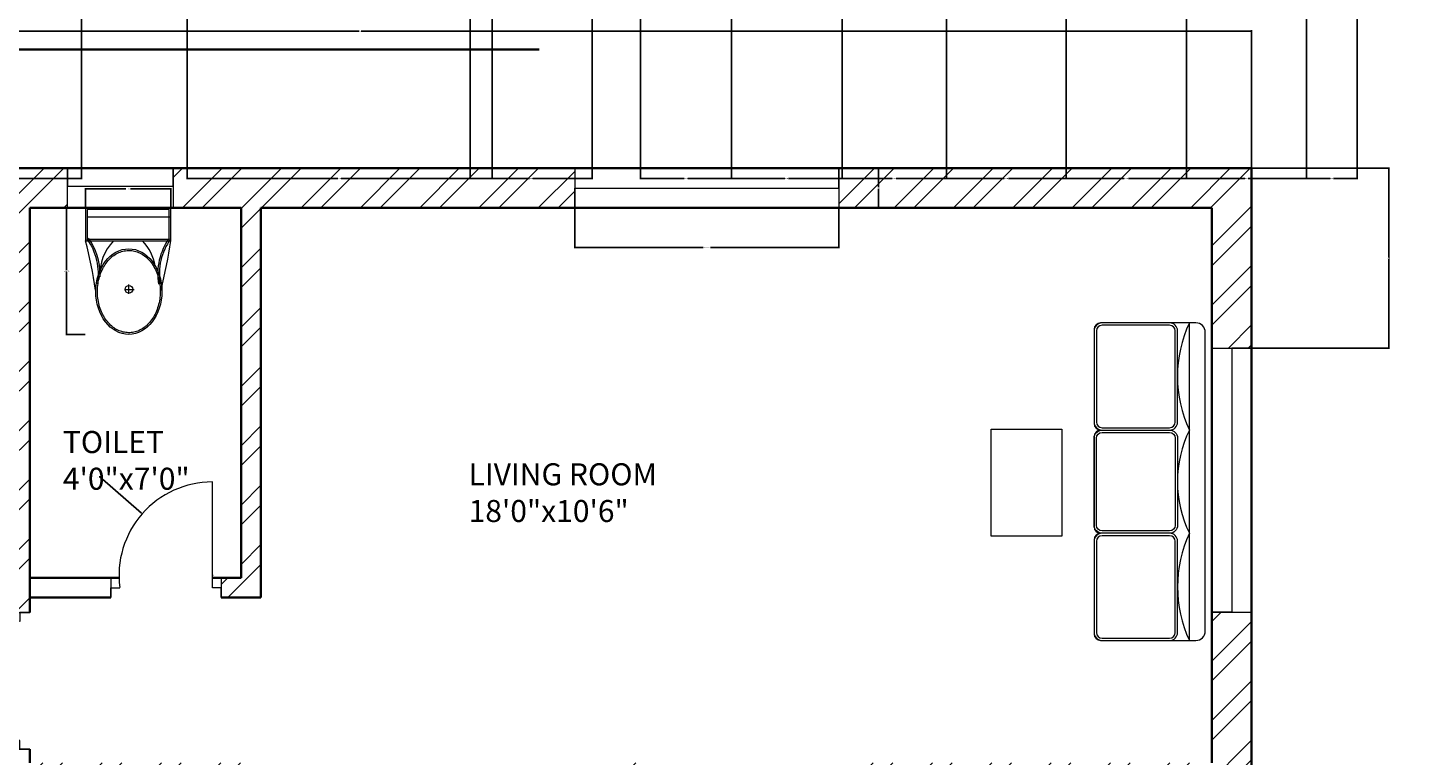
# Model space of a CAD drawing. Units: inches. Extents: x 1955 to 3324, y 980 to 3129.
# Tile 6 of 11: x 2237 to 2555, y 2323 to 2488. Entities that reach past the tile are written whole.
import ezdxf

# ---------------------------------------------------------------- set-up
doc = ezdxf.new("R2010")
doc.units = ezdxf.units.IN
for name, color, linetype, lineweight in [('A-ANNO-DIMS', 2, 'Continuous', 18), ('A-ANNO-TITL', 7, 'Continuous', 35), ('A-AREA-IDEN', 7, 'Continuous', 18), ('A-DOOR', 3, 'Continuous', 18), ('A-FLOR-FIXT', 9, 'Continuous', 18), ('A-FURN', 8, 'Continuous', 18), ('A-GLAZ', 4, 'Continuous', 18), ('A-WALL', 7, 'Continuous', 35), ('A-WALL-PATT', 252, 'Continuous', 13)]:
    doc.layers.add(name, color=color, linetype=linetype, lineweight=lineweight)
doc.styles.get("Standard").update_dxf_attribs({"font": 'arial.ttf'})
doc.dimstyles.get("Standard").update_dxf_attribs({"dimtxt": 0.18, "dimasz": 0.18, "dimexe": 0.18, "dimexo": 0.0625, "dimgap": 0.09, "dimtad": 0, "dimtih": 1, "dimtoh": 1, "dimdec": 4, "dimzin": 0, "dimdsep": 46, "dimtxsty": 'Standard', "dimcen": 0.09, "dimadec": 0, "dimazin": 0, "dimtfac": 1, "dimtdec": 4, "dimtofl": 0, "dimtmove": 0, "dimatfit": 3, "dimfxl": 1, "dimtolj": 1, "dimtzin": 0, "dimarcsym": 0})

# ---------------------------------------------------------------- blocks, each defined once
blk = doc.blocks.new('A$C31115884')
for p, q in [((257.5, 466.4), (257.5, 523.2)), ((283.1, 497.7), (223.4, 497.7)), ((0, 200), (0, 0)), ((520, 200), (0, 200)), ((10, 190), (10, 10)), ((510, 190), (10, 190)), ((510, 10), (510, 190)), ((520, 0), (520, 200)), ((510, 54.5), (0, 54.5)), ((10, 10), (510, 10)), ((0, 0), (520, 0))]:
    blk.add_line(p, q)
blk.add_circle((255.6, 496.4), 23.6)
for centre, radius, start, end in [((2777.7, -204.6), 2807, 165.4549, 171.71327), ((-294.5, 403.3), 364.7, 324.20913, 9.34987), ((-294.5, 403.3), 374.7, 324.20913, 9.34987), ((805.8, 403.3), 364.7, 170.65013, 215.79087), ((3237, 905), 2807, 188.28673, 194.5451), ((383.6, 406.2), 293.5, 190.27735, 224.15636), ((139.5, 406.2), 293.5, 315.84364, 2.65635), ((805.8, 403.3), 374.7, 179.20365, 215.79087)]:
    blk.add_arc(centre, radius, start, end)
blk.add_ellipse((256.2, 509.9), major_axis=(0, -260.7), ratio=0.772727)
blk.add_open_spline([(256.2, 259.2), (263.1, 259.2), (270, 259.7), (287.8, 262.3), (298.7, 265.1), (319.9, 273.1), (330.2, 278.4), (350.1, 291.1), (359.7, 298.7), (377.7, 315.9), (386.2, 325.5), (401.7, 346.6), (408.8, 358.1), (421.3, 382.5), (426.8, 395.5), (435.9, 422.4), (439.5, 436.4), (444.8, 465.1), (446.5, 479.7), (447.9, 509.2), (447.6, 524), (445, 553.3), (442.7, 567.8), (436.3, 596), (432.1, 609.7), (421.9, 636), (416, 648.6), (402.5, 672.1), (395, 683), (378.6, 703), (369.8, 712.1), (351.1, 728), (341.3, 734.8), (320.9, 746.2), (310.4, 750.7), (288.9, 757.3), (278, 759.4), (256, 761), (245, 760.6), (223.1, 757.2), (212.3, 754.3), (191.1, 746.1), (180.8, 740.7), (160.9, 727.8), (151.4, 720.1), (133.5, 702.7), (125.1, 693), (109.6, 671.7), (102.6, 660.2), (90.2, 635.7), (84.9, 622.7), (76, 595.6), (72.4, 581.6), (67.2, 552.9), (65.6, 538.2), (64.4, 508.8), (64.8, 494), (67.5, 464.7), (69.9, 450.2), (76.6, 422), (80.8, 408.3), (91.1, 382.2), (97.2, 369.7), (110.8, 346.3), (118.4, 335.4), (134.8, 315.6), (143.7, 306.7), (162.4, 290.9), (172.3, 284.2), (192.8, 273), (203.3, 268.6), (224.8, 262.2), (235.8, 260.2), (249.9, 259.3), (253, 259.2), (256.2, 259.2)], degree=3, knots=[0, 0, 0, 0, 0.110105, 0.110105, 0.285049, 0.285049, 0.459994, 0.459994, 0.634938, 0.634938, 0.809882, 0.809882, 0.984827, 0.984827, 1.159771, 1.159771, 1.334715, 1.334715, 1.50966, 1.50966, 1.684604, 1.684604, 1.859549, 1.859549, 2.034493, 2.034493, 2.209437, 2.209437, 2.384382, 2.384382, 2.559326, 2.559326, 2.73427, 2.73427, 2.909215, 2.909215, 3.084159, 3.084159, 3.259103, 3.259103, 3.434048, 3.434048, 3.608992, 3.608992, 3.783936, 3.783936, 3.958881, 3.958881, 4.133825, 4.133825, 4.30877, 4.30877, 4.483714, 4.483714, 4.658658, 4.658658, 4.833603, 4.833603, 5.008547, 5.008547, 5.183491, 5.183491, 5.358436, 5.358436, 5.53338, 5.53338, 5.708324, 5.708324, 5.883269, 5.883269, 6.058213, 6.058213, 6.233158, 6.233158, 6.283185, 6.283185, 6.283185, 6.283185])
blk = doc.blocks.new('COFFEE-TABLE-RECT')
blk.add_lwpolyline([(0, 24.35), (16.02, 24.35), (16.02, 0), (0, 0)], close=True)
blk = doc.blocks.new('DOOR-BED-N')
for p, q in [((33.75, 31.05), (38.25, 31.05)), ((38.25, 31.05), (36, 31.05)), ((36, 31.05), (36, 29.05)), ((36, 2), (0, 2)), ((36, 0), (36, 2)), ((33.75, 0), (38.25, 0)), ((38.25, 0), (36, 0))]:
    blk.add_line(p, q)
blk.add_arc((28.16, 2), 28.16, 73.8433, 180)
blk = doc.blocks.new('DOOR-WC-N')
for p, q in [((23.02, 2.25), (23.02, 26.25)), ((0, 4.5), (0, 0)), ((25.02, 4.5), (25.02, 0)), ((0, 0), (0, 2.25)), ((0, 2.25), (2, 2.25)), ((25.02, 2.25), (23.02, 2.25)), ((25.02, 0), (25.02, 2.25))]:
    blk.add_line(p, q)
blk.add_arc((23.02, 5.05), 21.2, 90, 187.5818)
blk = doc.blocks.new('WIN-PLAN-60-A')
for p, q in [((0, 60), (9, 60)), ((9, 60), (4.5, 60)), ((4.5, 60), (4.5, 0)), ((4.5, 0), (0, 0)), ((0, 0), (9, 0))]:
    blk.add_line(p, q)
blk = doc.blocks.new('WIN-PLAN-60-C')
for p, q in [((0, 9), (0, 0)), ((60, 4.5), (60, 9)), ((60, 9), (60, 9)), ((60, 9), (60, 0)), ((0, 0), (0, 4.5)), ((0, 4.5), (60, 4.5))]:
    blk.add_line(p, q)
blk = doc.blocks.new('WIN-PLAN-24-B')
for p, q in [((0, 0), (0, 9)), ((0, 9), (0, 4.93)), ((24, 4.93), (24, 9)), ((24, 9), (24, 0)), ((0, 4.93), (24, 4.93))]:
    blk.add_line(p, q)
blk = doc.blocks.new('*D35')
at = {"layer": 'A-ANNO-DIMS', "color": 0, "lineweight": -2, "transparency": 16777216}
for p, q in [((2361.48, 2447.44), (2361.48, 2438.32)), ((2421.48, 2447.44), (2421.48, 2438.32)), ((2361.66, 2438.5), (2390.63, 2438.5)), ((2421.3, 2438.5), (2392.32, 2438.5))]:
    blk.add_line(p, q, dxfattribs=at)
at = {"layer": 'A-ANNO-DIMS', "color": 0, "transparency": 16777216}
for points in [[(2361.66, 2438.53), (2361.66, 2438.47), (2361.48, 2438.5)], [(2421.3, 2438.53), (2421.3, 2438.47), (2421.48, 2438.5)]]:
    blk.add_solid(points, dxfattribs=at)
at = {"layer": 'Defpoints', "color": 0, "transparency": 16777216}
for p in [(2361.48, 2447.5), (2421.48, 2447.5), (2421.48, 2438.5)]:
    blk.add_point(p, dxfattribs=at)
at = {"layer": 'A-ANNO-DIMS', "color": 0, "transparency": 16777216, "insert": (2391.48, 2438.5), "char_height": 0.18, "attachment_point": 5}
blk.add_mtext('\\A1;WIN. 60 TYP.', dxfattribs=at)
blk = doc.blocks.new('*D36')
at = {"layer": 'A-ANNO-DIMS', "color": 0, "lineweight": -2, "transparency": 16777216}
for p, q in [((2421.54, 2456.5), (2430.66, 2456.5)), ((2430.48, 2456.32), (2430.48, 2452.19)), ((2430.48, 2447.68), (2430.48, 2451.82)), ((2421.54, 2447.5), (2430.66, 2447.5))]:
    blk.add_line(p, q, dxfattribs=at)
at = {"layer": 'A-ANNO-DIMS', "color": 0, "transparency": 16777216}
for points in [[(2430.45, 2456.32), (2430.51, 2456.32), (2430.48, 2456.5)], [(2430.45, 2447.68), (2430.51, 2447.68), (2430.48, 2447.5)]]:
    blk.add_solid(points, dxfattribs=at)
at = {"layer": 'Defpoints', "color": 0, "transparency": 16777216}
for p in [(2421.48, 2456.5), (2430.48, 2456.5), (2421.48, 2447.5)]:
    blk.add_point(p, dxfattribs=at)
at = {"layer": 'A-ANNO-DIMS', "color": 0, "transparency": 16777216, "insert": (2430.48, 2452), "char_height": 0.18, "attachment_point": 5}
blk.add_mtext('\\A1;9 TYP.', dxfattribs=at)
blk = doc.blocks.new('*D55')
at = {"layer": 'A-ANNO-DIMS', "color": 0, "lineweight": -2, "transparency": 16777216}
for p, q in [((2250.32, 2447.5), (2245.89, 2447.5)), ((2246.07, 2447.32), (2246.07, 2433.33)), ((2246.07, 2418.96), (2246.07, 2432.96)), ((2250.32, 2418.78), (2245.89, 2418.78))]:
    blk.add_line(p, q, dxfattribs=at)
at = {"layer": 'A-ANNO-DIMS', "color": 0, "transparency": 16777216}
for points in [[(2246.04, 2447.32), (2246.1, 2447.32), (2246.07, 2447.5)], [(2246.04, 2418.96), (2246.1, 2418.96), (2246.07, 2418.78)]]:
    blk.add_solid(points, dxfattribs=at)
at = {"layer": 'Defpoints', "color": 0, "transparency": 16777216}
for p in [(2250.38, 2447.5), (2246.07, 2418.78), (2250.38, 2418.78)]:
    blk.add_point(p, dxfattribs=at)
at = {"layer": 'A-ANNO-DIMS', "color": 0, "transparency": 16777216, "insert": (2246.07, 2433.14), "char_height": 0.18, "attachment_point": 5}
blk.add_mtext('\\A1;WC 29 TYP.', dxfattribs=at)
blk = doc.blocks.new('*D56')
at = {"layer": 'A-ANNO-DIMS', "color": 0, "lineweight": -2, "transparency": 16777216}
for p, q in [((2250.38, 2447.57), (2250.38, 2451.99)), ((2250.56, 2451.81), (2259.55, 2451.81)), ((2269.58, 2451.81), (2260.59, 2451.81)), ((2269.76, 2447.57), (2269.76, 2451.99))]:
    blk.add_line(p, q, dxfattribs=at)
at = {"layer": 'A-ANNO-DIMS', "color": 0, "transparency": 16777216}
for points in [[(2250.56, 2451.84), (2250.56, 2451.78), (2250.38, 2451.81)], [(2269.58, 2451.84), (2269.58, 2451.78), (2269.76, 2451.81)]]:
    blk.add_solid(points, dxfattribs=at)
at = {"layer": 'Defpoints', "color": 0, "transparency": 16777216}
for p in [(2250.38, 2451.81), (2250.38, 2447.5), (2269.76, 2447.5)]:
    blk.add_point(p, dxfattribs=at)
at = {"layer": 'A-ANNO-DIMS', "color": 0, "transparency": 16777216, "insert": (2260.07, 2451.81), "char_height": 0.18, "attachment_point": 5}
blk.add_mtext('\\A1;19 TYP.', dxfattribs=at)
blk = doc.blocks.new('*D91')
at = {"layer": 'A-ANNO-DIMS', "color": 0, "lineweight": -2, "transparency": 16777216}
for p, q in [((2110.21, 2456.57), (2110.21, 2487.83)), ((2110.39, 2487.65), (2312.42, 2487.65)), ((2515.03, 2487.65), (2313, 2487.65)), ((2515.21, 2456.57), (2515.21, 2487.83))]:
    blk.add_line(p, q, dxfattribs=at)
at = {"layer": 'A-ANNO-DIMS', "color": 0, "transparency": 16777216}
for points in [[(2110.39, 2487.68), (2110.39, 2487.62), (2110.21, 2487.65)], [(2515.03, 2487.68), (2515.03, 2487.62), (2515.21, 2487.65)]]:
    blk.add_solid(points, dxfattribs=at)
at = {"layer": 'Defpoints', "color": 0, "transparency": 16777216}
for p in [(2515.21, 2487.65), (2110.21, 2456.5), (2515.21, 2456.5)]:
    blk.add_point(p, dxfattribs=at)
at = {"layer": 'A-ANNO-DIMS', "color": 0, "transparency": 16777216, "insert": (2312.71, 2487.65), "char_height": 0.18, "attachment_point": 5}
blk.add_mtext('\\A1;405', dxfattribs=at)
blk = doc.blocks.new('*D106')
at = {"layer": 'A-ANNO-DIMS', "color": 0, "lineweight": -2, "transparency": 16777216}
for p, q in [((2515.27, 2456.5), (2546.54, 2456.5)), ((2546.36, 2456.32), (2546.36, 2436.27)), ((2546.36, 2415.84), (2546.36, 2435.9)), ((2515.27, 2415.66), (2546.54, 2415.66))]:
    blk.add_line(p, q, dxfattribs=at)
at = {"layer": 'A-ANNO-DIMS', "color": 0, "transparency": 16777216}
for points in [[(2546.33, 2456.32), (2546.39, 2456.32), (2546.36, 2456.5)], [(2546.33, 2415.84), (2546.39, 2415.84), (2546.36, 2415.66)]]:
    blk.add_solid(points, dxfattribs=at)
at = {"layer": 'Defpoints', "color": 0, "transparency": 16777216}
for p in [(2515.21, 2456.5), (2546.36, 2456.5), (2515.21, 2415.66)]:
    blk.add_point(p, dxfattribs=at)
at = {"layer": 'A-ANNO-DIMS', "color": 0, "transparency": 16777216, "insert": (2546.36, 2436.08), "char_height": 0.18, "attachment_point": 5}
blk.add_mtext('\\A1;40.84', dxfattribs=at)
blk = doc.blocks.new('*D116')
at = {"layer": 'A-ANNO-DIMS', "color": 0, "lineweight": -2, "transparency": 16777216}
for p, q in [((2206.36, 2610.35), (2206.36, 2454)), ((2249.49, 2610.35), (2249.49, 2454)), ((2206.54, 2454.18), (2227.53, 2454.18)), ((2249.31, 2454.18), (2228.32, 2454.18))]:
    blk.add_line(p, q, dxfattribs=at)
at = {"layer": 'A-ANNO-DIMS', "color": 0, "transparency": 16777216}
for points in [[(2206.54, 2454.21), (2206.54, 2454.15), (2206.36, 2454.18)], [(2249.31, 2454.21), (2249.31, 2454.15), (2249.49, 2454.18)]]:
    blk.add_solid(points, dxfattribs=at)
at = {"layer": 'Defpoints', "color": 0, "transparency": 16777216}
for p in [(2206.36, 2610.41), (2249.49, 2610.41), (2249.49, 2454.18)]:
    blk.add_point(p, dxfattribs=at)
at = {"layer": 'A-ANNO-DIMS', "color": 0, "transparency": 16777216, "insert": (2227.93, 2454.18), "char_height": 0.18, "attachment_point": 5}
blk.add_mtext('\\A1;43.13', dxfattribs=at)
blk = doc.blocks.new('*D117')
at = {"layer": 'A-ANNO-DIMS', "color": 0, "lineweight": -2, "transparency": 16777216}
for p, q in [((2273.49, 2610.35), (2273.49, 2454)), ((2342.7, 2610.35), (2342.7, 2454)), ((2273.67, 2454.18), (2307.72, 2454.18)), ((2342.52, 2454.18), (2308.47, 2454.18))]:
    blk.add_line(p, q, dxfattribs=at)
at = {"layer": 'A-ANNO-DIMS', "color": 0, "transparency": 16777216}
for points in [[(2273.67, 2454.21), (2273.67, 2454.15), (2273.49, 2454.18)], [(2342.52, 2454.21), (2342.52, 2454.15), (2342.7, 2454.18)]]:
    blk.add_solid(points, dxfattribs=at)
at = {"layer": 'Defpoints', "color": 0, "transparency": 16777216}
for p in [(2273.49, 2610.41), (2342.7, 2610.41), (2342.7, 2454.18)]:
    blk.add_point(p, dxfattribs=at)
at = {"layer": 'A-ANNO-DIMS', "color": 0, "transparency": 16777216, "insert": (2308.09, 2454.18), "char_height": 0.18, "attachment_point": 5}
blk.add_mtext('\\A1;69.21', dxfattribs=at)
blk = doc.blocks.new('*D123')
at = {"layer": 'A-ANNO-DIMS', "color": 0, "lineweight": -2, "transparency": 16777216}
for p, q in [((2337.77, 3041.34), (2337.77, 2454)), ((2365.46, 3041.34), (2365.46, 2454)), ((2337.95, 2454.18), (2351.22, 2454.18)), ((2365.28, 2454.18), (2352.01, 2454.18))]:
    blk.add_line(p, q, dxfattribs=at)
at = {"layer": 'A-ANNO-DIMS', "color": 0, "transparency": 16777216}
for points in [[(2337.95, 2454.21), (2337.95, 2454.15), (2337.77, 2454.18)], [(2365.28, 2454.21), (2365.28, 2454.15), (2365.46, 2454.18)]]:
    blk.add_solid(points, dxfattribs=at)
at = {"layer": 'Defpoints', "color": 0, "transparency": 16777216}
for p in [(2337.77, 3041.4), (2365.46, 3041.4), (2365.46, 2454.18)]:
    blk.add_point(p, dxfattribs=at)
at = {"layer": 'A-ANNO-DIMS', "color": 0, "transparency": 16777216, "insert": (2351.62, 2454.18), "char_height": 0.18, "attachment_point": 5}
blk.add_mtext('\\A1;27.69', dxfattribs=at)
blk = doc.blocks.new('*D124')
at = {"layer": 'A-ANNO-DIMS', "color": 0, "lineweight": -2, "transparency": 16777216}
for p, q in [((2376.45, 2978.61), (2376.45, 2454)), ((2397.08, 2978.61), (2397.08, 2454)), ((2376.63, 2454.18), (2386.37, 2454.18)), ((2396.9, 2454.18), (2387.16, 2454.18))]:
    blk.add_line(p, q, dxfattribs=at)
at = {"layer": 'A-ANNO-DIMS', "color": 0, "transparency": 16777216}
for points in [[(2376.63, 2454.21), (2376.63, 2454.15), (2376.45, 2454.18)], [(2396.9, 2454.21), (2396.9, 2454.15), (2397.08, 2454.18)]]:
    blk.add_solid(points, dxfattribs=at)
at = {"layer": 'Defpoints', "color": 0, "transparency": 16777216}
for p in [(2376.45, 2978.67), (2397.08, 2978.67), (2397.08, 2454.18)]:
    blk.add_point(p, dxfattribs=at)
at = {"layer": 'A-ANNO-DIMS', "color": 0, "transparency": 16777216, "insert": (2386.76, 2454.18), "char_height": 0.18, "attachment_point": 5}
blk.add_mtext('\\A1;20.63', dxfattribs=at)
blk = doc.blocks.new('*D125')
at = {"layer": 'A-ANNO-DIMS', "color": 0, "lineweight": -2, "transparency": 16777216}
for p, q in [((2397.08, 2978.61), (2397.08, 2454)), ((2422.2, 2978.61), (2422.2, 2454)), ((2397.26, 2454.18), (2409.24, 2454.18)), ((2422.02, 2454.18), (2410.03, 2454.18))]:
    blk.add_line(p, q, dxfattribs=at)
at = {"layer": 'A-ANNO-DIMS', "color": 0, "transparency": 16777216}
for points in [[(2397.26, 2454.21), (2397.26, 2454.15), (2397.08, 2454.18)], [(2422.02, 2454.21), (2422.02, 2454.15), (2422.2, 2454.18)]]:
    blk.add_solid(points, dxfattribs=at)
at = {"layer": 'Defpoints', "color": 0, "transparency": 16777216}
for p in [(2397.08, 2978.67), (2422.2, 2978.67), (2422.2, 2454.18)]:
    blk.add_point(p, dxfattribs=at)
at = {"layer": 'A-ANNO-DIMS', "color": 0, "transparency": 16777216, "insert": (2409.64, 2454.18), "char_height": 0.18, "attachment_point": 5}
blk.add_mtext('\\A1;25.12', dxfattribs=at)
blk = doc.blocks.new('*D126')
at = {"layer": 'A-ANNO-DIMS', "color": 0, "lineweight": -2, "transparency": 16777216}
for p, q in [((2422.2, 2978.61), (2422.2, 2454)), ((2445.92, 2978.61), (2445.92, 2454)), ((2422.38, 2454.18), (2433.59, 2454.18)), ((2445.74, 2454.18), (2434.52, 2454.18))]:
    blk.add_line(p, q, dxfattribs=at)
at = {"layer": 'A-ANNO-DIMS', "color": 0, "transparency": 16777216}
for points in [[(2422.38, 2454.21), (2422.38, 2454.15), (2422.2, 2454.18)], [(2445.74, 2454.21), (2445.74, 2454.15), (2445.92, 2454.18)]]:
    blk.add_solid(points, dxfattribs=at)
at = {"layer": 'Defpoints', "color": 0, "transparency": 16777216}
for p in [(2422.2, 2978.67), (2445.92, 2978.67), (2445.92, 2454.18)]:
    blk.add_point(p, dxfattribs=at)
at = {"layer": 'A-ANNO-DIMS', "color": 0, "transparency": 16777216, "insert": (2434.06, 2454.18), "char_height": 0.18, "attachment_point": 5}
blk.add_mtext('\\A1;23.727', dxfattribs=at)
blk = doc.blocks.new('*D127')
at = {"layer": 'A-ANNO-DIMS', "color": 0, "lineweight": -2, "transparency": 16777216}
for p, q in [((2445.92, 2978.61), (2445.92, 2454)), ((2473.12, 2978.61), (2473.12, 2454)), ((2446.1, 2454.18), (2459.05, 2454.18)), ((2472.94, 2454.18), (2459.99, 2454.18))]:
    blk.add_line(p, q, dxfattribs=at)
at = {"layer": 'A-ANNO-DIMS', "color": 0, "transparency": 16777216}
for points in [[(2446.1, 2454.21), (2446.1, 2454.15), (2445.92, 2454.18)], [(2472.94, 2454.21), (2472.94, 2454.15), (2473.12, 2454.18)]]:
    blk.add_solid(points, dxfattribs=at)
at = {"layer": 'Defpoints', "color": 0, "transparency": 16777216}
for p in [(2445.92, 2978.67), (2473.12, 2978.67), (2473.12, 2454.18)]:
    blk.add_point(p, dxfattribs=at)
at = {"layer": 'A-ANNO-DIMS', "color": 0, "transparency": 16777216, "insert": (2459.52, 2454.18), "char_height": 0.18, "attachment_point": 5}
blk.add_mtext('\\A1;27.195', dxfattribs=at)
blk = doc.blocks.new('*D128')
at = {"layer": 'A-ANNO-DIMS', "color": 0, "lineweight": -2, "transparency": 16777216}
for p, q in [((2473.12, 2978.61), (2473.12, 2454)), ((2500.43, 2978.61), (2500.43, 2454)), ((2473.3, 2454.18), (2486.31, 2454.18)), ((2500.25, 2454.18), (2487.24, 2454.18))]:
    blk.add_line(p, q, dxfattribs=at)
at = {"layer": 'A-ANNO-DIMS', "color": 0, "transparency": 16777216}
for points in [[(2473.3, 2454.21), (2473.3, 2454.15), (2473.12, 2454.18)], [(2500.25, 2454.21), (2500.25, 2454.15), (2500.43, 2454.18)]]:
    blk.add_solid(points, dxfattribs=at)
at = {"layer": 'Defpoints', "color": 0, "transparency": 16777216}
for p in [(2473.12, 2978.67), (2500.43, 2978.67), (2500.43, 2454.18)]:
    blk.add_point(p, dxfattribs=at)
at = {"layer": 'A-ANNO-DIMS', "color": 0, "transparency": 16777216, "insert": (2486.77, 2454.18), "char_height": 0.18, "attachment_point": 5}
blk.add_mtext('\\A1;27.314', dxfattribs=at)
blk = doc.blocks.new('*D129')
at = {"layer": 'A-ANNO-DIMS', "color": 0, "lineweight": -2, "transparency": 16777216}
for p, q in [((2500.43, 2978.61), (2500.43, 2454)), ((2527.66, 2978.61), (2527.66, 2454)), ((2500.61, 2454.18), (2513.65, 2454.18)), ((2527.48, 2454.18), (2514.44, 2454.18))]:
    blk.add_line(p, q, dxfattribs=at)
at = {"layer": 'A-ANNO-DIMS', "color": 0, "transparency": 16777216}
for points in [[(2500.61, 2454.21), (2500.61, 2454.15), (2500.43, 2454.18)], [(2527.48, 2454.21), (2527.48, 2454.15), (2527.66, 2454.18)]]:
    blk.add_solid(points, dxfattribs=at)
at = {"layer": 'Defpoints', "color": 0, "transparency": 16777216}
for p in [(2500.43, 2978.67), (2527.66, 2978.67), (2527.66, 2454.18)]:
    blk.add_point(p, dxfattribs=at)
at = {"layer": 'A-ANNO-DIMS', "color": 0, "transparency": 16777216, "insert": (2514.05, 2454.18), "char_height": 0.18, "attachment_point": 5}
blk.add_mtext('\\A1;27.23', dxfattribs=at)
blk = doc.blocks.new('*D130')
at = {"layer": 'A-ANNO-DIMS', "color": 0, "lineweight": -2, "transparency": 16777216}
for p, q in [((2539.21, 3060.35), (2539.21, 2454)), ((2527.66, 3047.91), (2527.66, 2454)), ((2527.84, 2454.18), (2533.05, 2454.18)), ((2539.03, 2454.18), (2533.82, 2454.18))]:
    blk.add_line(p, q, dxfattribs=at)
at = {"layer": 'A-ANNO-DIMS', "color": 0, "transparency": 16777216}
for points in [[(2527.84, 2454.21), (2527.84, 2454.15), (2527.66, 2454.18)], [(2539.03, 2454.21), (2539.03, 2454.15), (2539.21, 2454.18)]]:
    blk.add_solid(points, dxfattribs=at)
at = {"layer": 'Defpoints', "color": 0, "transparency": 16777216}
for p in [(2539.21, 3060.41), (2527.66, 3047.98), (2539.21, 2454.18)]:
    blk.add_point(p, dxfattribs=at)
at = {"layer": 'A-ANNO-DIMS', "color": 0, "transparency": 16777216, "insert": (2533.44, 2454.18), "char_height": 0.18, "attachment_point": 5}
blk.add_mtext('\\A1;11.55', dxfattribs=at)
blk = doc.blocks.new('*D145')
at = {"layer": 'A-ANNO-DIMS', "color": 0, "lineweight": -2, "transparency": 16777216}
for p, q in [((2253.48, 2386.4), (2253.66, 2386.4)), ((2253.66, 2386.4), (2263.09, 2378.14)), ((2279.09, 2364.05), (2279.27, 2364.05)), ((2279.18, 2363.96), (2279.18, 2364.14))]:
    blk.add_line(p, q, dxfattribs=at)
at = {"layer": 'A-ANNO-DIMS', "color": 0, "transparency": 16777216}
blk.add_solid([(2263.11, 2378.16), (2263.07, 2378.12), (2263.23, 2378.02)], dxfattribs=at)
at = {"layer": 'Defpoints', "color": 0, "transparency": 16777216}
for p in [(2263.23, 2378.02), (2279.18, 2364.05)]:
    blk.add_point(p, dxfattribs=at)
at = {"layer": 'A-ANNO-DIMS', "color": 0, "transparency": 16777216, "insert": (2252.93, 2386.4), "char_height": 0.18, "attachment_point": 5}
blk.add_mtext('\\A1;R21.203', dxfattribs=at)

msp = doc.modelspace()

# ---------------------------------------------------------------- hatches: boundary and pattern name
at = {"layer": 'A-WALL-PATT'}
h = msp.add_hatch(dxfattribs=at)
h.set_pattern_fill('ANSI32', color=256)
h.paths.add_polyline_path([(2361.4775, 2456.5037), (2270.2755, 2456.5037), (2270.2755, 2447.5037), (2285.7102, 2447.5037), (2285.7102, 2363.5037), (2281.1795, 2363.5037), (2281.1795, 2359.0037), (2290.2102, 2359.0037), (2290.2102, 2447.5037), (2361.4775, 2447.5037), (2361.4775, 2452.0037)])
h.paths.add_polyline_path([(2246.2755, 2456.5037), (2197.6809, 2456.5037), (2197.6809, 2447.5037), (2233.2102, 2447.5037), (2233.2102, 2355.6044), (2237.7102, 2355.6044), (2237.7102, 2447.5037), (2246.2755, 2447.5037)], flags=17)
h.paths.add_polyline_path([(2137.6809, 2456.5037), (2110.2102, 2456.5037), (2110.2102, 2312.5037), (2152.2102, 2312.5037), (2281.2102, 2312.5037), (2281.2102, 2107.6185), (2290.2102, 2107.6185), (2290.2102, 2267.9289), (2329.216, 2267.9289), (2329.216, 2272.4289), (2329.216, 2276.9289), (2290.2102, 2276.9289), (2290.2102, 2321.5037), (2281.2102, 2321.5037), (2119.2102, 2321.5037), (2119.2102, 2447.5037), (2137.6809, 2447.5037)])
h.paths.add_polyline_path([(2515.2102, 2456.5037), (2421.4775, 2456.5037), (2421.4775, 2447.5037), (2506.2102, 2447.5037), (2506.2102, 2415.6626), (2515.2102, 2415.6626)])
h.paths.add_polyline_path([(2515.2102, 2355.6626), (2506.2102, 2355.6626), (2506.2102, 2321.5037), (2424.9282, 2321.5037), (2424.9282, 2312.5037), (2461.2102, 2312.5037), (2470.2102, 2312.5037), (2515.2102, 2312.5037)])
h.paths.add_polyline_path([(2515.2102, 2232.5037), (2470.2102, 2232.5037), (2470.2102, 2237.3759), (2465.7102, 2237.3759), (2461.2102, 2237.3759), (2461.2102, 2232.5037), (2377.2219, 2232.5037), (2377.2219, 2321.5037), (2368.2219, 2321.5037), (2368.2219, 2276.9289), (2359.3802, 2276.9289), (2359.3802, 2272.4289), (2359.3802, 2267.9289), (2368.2219, 2267.9289), (2368.2219, 2223.5037), (2377.2219, 2223.5037), (2461.2102, 2223.5037), (2506.2102, 2223.5037), (2506.2102, 2129.5037), (2461.2102, 2129.5037), (2387.2102, 2129.5037), (2368.2219, 2129.5037), (2368.2219, 2056.4936), (2361.0095, 2056.4936), (2361.0095, 2051.9936), (2361.0095, 2047.4936), (2368.2219, 2047.4936), (2368.2219, 2031.5037), (2377.2219, 2031.5037), (2377.2219, 2120.5037), (2461.2102, 2120.5037), (2461.2102, 2112.7921), (2470.2102, 2112.7921), (2470.2102, 2120.5037), (2515.2102, 2120.5037), (2515.2102, 2129.5037)])
h.paths.add_polyline_path([(2470.2102, 2277.1758), (2461.2102, 2277.1758), (2461.2102, 2272.5037), (2461.2102, 2270.2549), (2470.2102, 2270.2549), (2470.2102, 2272.5037)], flags=17)
h.paths.add_polyline_path([(2515.2102, 2040.5037), (2470.2102, 2040.5037), (2417.8264, 2040.5037), (2417.8264, 2031.5037), (2506.2102, 2031.5037), (2506.2102, 2005.3639), (2515.2102, 2005.3639)])
h.paths.add_polyline_path([(2506.2102, 1905.5037), (2402.6963, 1905.5037), (2402.6963, 1896.5037), (2506.2102, 1896.5037)])
h.paths.add_polyline_path([(2515.2102, 1945.3639), (2506.2102, 1945.3639), (2506.2102, 1905.5037), (2506.2102, 1896.5037), (2515.2102, 1896.5037)])
h.paths.add_polyline_path([(2342.6963, 1901.0037), (2342.6963, 1905.5037), (2273.4892, 1905.5037), (2273.4892, 1896.5037), (2342.6963, 1896.5037)])
h.paths.add_polyline_path([(2290.2102, 1994.0037), (2283.612, 1994.0037), (2283.612, 1991.7537), (2283.612, 1989.5037), (2285.7102, 1989.5037), (2285.7102, 1905.5037), (2290.2102, 1905.5037)])
h.paths.add_polyline_path([(2249.4892, 1905.5037), (2237.7102, 1905.5037), (2206.3617, 1905.5037), (2206.3617, 1896.5037), (2249.4892, 1896.5037), (2249.4892, 1901.0037)])
h.paths.add_polyline_path([(2237.7102, 1989.5037), (2261.7102, 1989.5037), (2261.7102, 1994.0037), (2237.7102, 1994.0037), (2237.7102, 1999.266), (2235.4602, 1999.266), (2233.2102, 1999.266), (2233.2102, 1994.0037), (2233.2102, 1905.5037), (2237.7102, 1905.5037)])
h.paths.add_polyline_path([(2119.2102, 1947.5144), (2110.2102, 1947.5144), (2110.2102, 1896.5037), (2119.2102, 1896.5037), (2146.3617, 1896.5037), (2146.3617, 1901.0037), (2146.3617, 1905.5037), (2119.2102, 1905.5037)])
h.paths.add_polyline_path([(2119.2102, 2068.6379), (2110.2102, 2068.6379), (2110.2102, 2007.5144), (2119.2102, 2007.5144), (2119.2102, 2031.5037), (2233.2102, 2031.5037), (2233.2102, 2027.9287), (2235.4602, 2027.9287), (2237.7102, 2027.9287), (2237.7102, 2031.5037), (2281.2102, 2031.5037), (2290.2102, 2031.5037), (2290.2102, 2047.4936), (2326.409, 2047.4936), (2326.409, 2056.4936), (2290.2102, 2056.4936), (2290.2102, 2071.2722), (2285.7102, 2071.2722), (2281.2102, 2071.2722), (2281.2102, 2040.5037), (2227.2102, 2040.5037), (2227.2102, 2111.2571), (2222.7102, 2111.2571), (2218.2102, 2111.2571), (2218.2102, 2040.5037), (2119.2102, 2040.5037)])
h.paths.add_polyline_path([(2236.9166, 2214.5037), (2161.2102, 2214.5037), (2161.2102, 2221.6488), (2152.2102, 2221.6488), (2152.2102, 2214.5037), (2110.2102, 2214.5037), (2110.2102, 2205.5037), (2131.2394, 2205.5037), (2131.2394, 2198.3478), (2140.2394, 2198.3478), (2140.2394, 2205.5037), (2224.2394, 2205.5037), (2224.2394, 2200.2317), (2228.7394, 2200.2317), (2233.2394, 2200.2317), (2233.2394, 2205.5037), (2236.9166, 2205.5037)], flags=17)
h.paths.add_polyline_path([(2236.9166, 2157.5037), (2233.2394, 2157.5037), (2233.2394, 2178.9172), (2228.7394, 2178.9172), (2224.2394, 2178.9172), (2224.2394, 2157.5037), (2140.2394, 2157.5037), (2140.2394, 2174.3478), (2131.2394, 2174.3478), (2131.2394, 2157.5037), (2110.2102, 2157.5037), (2110.2102, 2128.6379), (2119.2102, 2128.6379), (2119.2102, 2148.5037), (2218.2102, 2148.5037), (2218.2102, 2141.7262), (2222.7102, 2141.7262), (2227.2102, 2141.7262), (2227.2102, 2148.5037), (2236.9166, 2148.5037)], flags=0)
h.paths.add_polyline_path([(3084.7449, 2537.3808), (3212.7954, 2537.3808), (3212.7954, 2555.9271), (3084.7449, 2555.9271)], flags=9)
h.paths.add_polyline_path([(3068.7485, 2853.43), (3169.977, 2853.43), (3169.977, 2871.9764), (3068.7485, 2871.9764)], flags=9)
h.paths.add_polyline_path([(3074.1798, 2918.0252), (3126.4732, 2918.0252), (3126.4732, 2936.5716), (3074.1798, 2936.5716)], flags=9)
h.paths.add_polyline_path([(3073.0928, 2947.3127), (3199.0499, 2947.3127), (3199.0499, 2965.8591), (3073.0928, 2965.8591)], flags=9)
h.paths.add_polyline_path([(2733.8393, 2484.8678), (2879.7915, 2484.8678), (2879.7915, 2521.9606), (2733.8393, 2521.9606)], flags=9)
h.paths.add_polyline_path([(2204.9881, 2482.4168), (2355.1272, 2482.4168), (2355.1272, 2519.5095), (2204.9881, 2519.5095)], flags=9)
h.paths.add_polyline_path([(3062.1429, 2387.2466), (3079.3735, 2387.2466), (3079.3735, 2411.9751), (3062.1429, 2411.9751)], flags=9)
h.paths.add_polyline_path([(2190.1574, 2158.8439), (2219.315, 2158.8439), (2219.315, 2177.5013), (2190.1574, 2177.5013)], flags=25)
h.paths.add_polyline_path([(2213.6766, 1840.7276), (2405.0382, 1840.7276), (2405.0382, 1865.4561), (2213.6766, 1865.4561)], flags=9)
h.paths.add_polyline_path([(2180.5398, 2233.911), (2213.9471, 2233.911), (2213.9471, 2252.5683), (2180.5398, 2252.5683)], flags=25)
h.paths.add_polyline_path([(2134.4484, 2238.3973), (2134.4484, 2274.2807), (2115.791, 2274.2807), (2115.791, 2238.3973)], flags=25)
h.paths.add_polyline_path([(2135.1593, 2122.9991), (2173.7507, 2122.9991), (2173.7507, 2141.6565), (2135.1593, 2141.6565)], flags=25)
h.paths.add_polyline_path([(2129.8822, 2002.1912), (2168.4736, 2002.1912), (2168.4736, 2020.8486), (2129.8822, 2020.8486)], flags=9)
h.paths.add_polyline_path([(2239.6647, 1953.4107), (2268.8973, 1953.4107), (2268.8973, 1972.068), (2239.6647, 1972.068)], flags=9)
h.paths.add_polyline_path([(2352.8562, 1951.2904), (2402.1775, 1951.2904), (2402.1775, 1969.9477), (2352.8562, 1969.9477)], flags=9)
h.paths.add_polyline_path([(2500.1358, 2055.32), (2500.1358, 2091.2034), (2481.4784, 2091.2034), (2481.4784, 2055.32)], flags=25)
h.paths.add_polyline_path([(2391.2702, 2058.6821), (2424.4285, 2058.6821), (2424.4285, 2077.3394), (2391.2702, 2077.3394)], flags=25)
h.paths.add_polyline_path([(2507.7996, 2257.2758), (2507.7996, 2293.1592), (2489.1422, 2293.1592), (2489.1422, 2257.2758)], flags=25)
h.paths.add_polyline_path([(2386.8349, 2273.8734), (2419.9931, 2273.8734), (2419.9931, 2292.5307), (2386.8349, 2292.5307)], flags=25)
h.paths.add_polyline_path([(2335.374, 2373.3267), (2384.6953, 2373.3267), (2384.6953, 2391.984), (2335.374, 2391.984)], flags=9)
h.paths.add_polyline_path([(2243.8205, 2380.6539), (2273.0531, 2380.6539), (2273.0531, 2399.3113), (2243.8205, 2399.3113)], flags=25)
h.paths.add_polyline_path([(2126.2627, 2321.6894), (2164.8541, 2321.6894), (2164.8541, 2340.3467), (2126.2627, 2340.3467)], flags=25)

# ---------------------------------------------------------------- linework, layer by layer
at = {"layer": 'A-ANNO-TITL'}
msp.add_line((2205.5822, 2483.435), (2353.4472, 2483.435), dxfattribs=at)
at = {"layer": 'A-FURN'}
for points in [[(2481.267, 2397.0465), (2496.5952, 2397.0465, 0.41421356), (2498.3986, 2398.8498), (2498.3986, 2419.588, 0.41421356), (2496.5952, 2421.3913), (2481.267, 2421.3913, 0.41421356), (2479.4637, 2419.588), (2479.4637, 2398.8498, 0.41421356)], [(2481.267, 2397.5875), (2496.5952, 2397.5875, 0.41421356), (2497.8576, 2398.8498), (2497.8576, 2419.588, 0.41421356), (2496.5952, 2420.8503), (2481.267, 2420.8503, 0.41421356), (2480.0047, 2419.588), (2480.0047, 2398.8498, 0.41421356)], [(2481.267, 2397.0465), (2496.5952, 2397.0465, -0.41421356), (2498.3986, 2395.2432), (2498.3986, 2375.4066, -0.41421356), (2496.5952, 2373.6033), (2481.267, 2373.6033, -0.41421356), (2479.4637, 2375.4066), (2479.4637, 2395.2432, -0.41421356)], [(2481.267, 2396.5055), (2496.5952, 2396.5055, -0.41421356), (2497.8576, 2395.2432), (2497.8576, 2375.4066, -0.41421356), (2496.5952, 2374.1443), (2481.267, 2374.1443, -0.41421356), (2480.0047, 2375.4066), (2480.0047, 2395.2432, -0.41421356)], [(2481.267, 2349.2585), (2496.5952, 2349.2585, 0.41421356), (2498.3986, 2351.0618), (2498.3986, 2371.8, 0.41421356), (2496.5952, 2373.6033), (2481.267, 2373.6033, 0.41421356), (2479.4637, 2371.8), (2479.4637, 2351.0618, 0.41421356)], [(2481.267, 2349.7995), (2496.5952, 2349.7995, 0.41421356), (2497.8576, 2351.0618), (2497.8576, 2371.8, 0.41421356), (2496.5952, 2373.0623), (2481.267, 2373.0623, 0.41421356), (2480.0047, 2371.8), (2480.0047, 2351.0618, 0.41421356)]]:
    msp.add_lwpolyline(points, format="xyb", close=True, dxfattribs=at)
at = {"layer": 'A-FURN', "ltscale": 0.03}
msp.add_lwpolyline([(2479.4637, 2372.1429), (2479.4637, 2350.7011, 0.41421356), (2480.9063, 2349.2585), (2502.5462, 2349.2585, 0.41421356), (2504.7102, 2351.4225), (2504.7102, 2419.2273, 0.41421356), (2502.5462, 2421.3913), (2480.9063, 2421.3913, 0.41421356), (2479.4637, 2419.9486), (2479.4637, 2398.5069, 0.41421356), (2480.9063, 2397.0642, -1), (2480.9063, 2397.0287, 0.41421356), (2479.4637, 2395.5861), (2479.4637, 2375.0637, 0.41421356), (2480.9063, 2373.621, -1), (2480.9063, 2373.5856, 0.41421356)], format="xyb", close=True, dxfattribs=at)
at = {"layer": 'A-FURN'}
msp.add_lwpolyline([(2501.1035, 2349.2585), (2501.1035, 2421.3913)], dxfattribs=at)
for centre, radius, start, end in [((2526.8009, 2409.2189), 28.4345, 154.653824, 205.346176), ((2524.9975, 2385.3249), 26.6143, 153.868999, 206.131001), ((2527.1014, 2361.4309), 28.7064, 154.910626, 205.089374)]:
    msp.add_arc(centre, radius, start, end, dxfattribs=at)
at = {"layer": 'A-WALL'}
for p, q in [((2110.2102, 2456.5037), (2515.2102, 2456.5037)), ((2515.2102, 2456.5037), (2515.2102, 1896.5037)), ((2237.7102, 2447.5037), (2237.7102, 2355.6044)), ((2237.7102, 2447.5037), (2285.7102, 2447.5037)), ((2285.7102, 2447.5037), (2285.7102, 2363.5037)), ((2290.2102, 2447.5037), (2290.2102, 2359.0037)), ((2290.2102, 2447.5037), (2506.2102, 2447.5037)), ((2506.2102, 2447.5037), (2506.2102, 2321.5037)), ((2237.7102, 2363.5037), (2257.9841, 2363.5037)), ((2279.1795, 2363.5037), (2285.7102, 2363.5037)), ((2237.7102, 2359.0037), (2256.1624, 2359.0037)), ((2281.1795, 2359.0037), (2290.2102, 2359.0037)), ((2237.7102, 2324.5535), (2237.7102, 2321.5037))]:
    msp.add_line(p, q, dxfattribs=at)

# ---------------------------------------------------------------- block references
at = {"layer": 'A-DOOR'}
for name, p in [('DOOR-WC-N', (2256.162, 2359.004)), ('DOOR-BED-N', (2199.46, 2324.554))]:
    msp.add_blockref(name, p, dxfattribs=at)
at = {"layer": 'A-FLOR-FIXT', "xscale": 0.0372717239612423, "yscale": 0.0372717239612423, "zscale": 0.0372717239612423, "rotation": 180}
msp.add_blockref('A$C31115884', (2269.7595, 2447.5037), dxfattribs=at)
at = {"layer": 'A-FURN'}
msp.add_blockref('COFFEE-TABLE-RECT', (2456.067, 2372.9388), dxfattribs=at)
at = {"layer": 'A-GLAZ'}
for name, p in [('WIN-PLAN-24-B', (2246.275, 2447.504)), ('WIN-PLAN-60-C', (2361.478, 2447.504)), ('WIN-PLAN-60-A', (2506.21, 2355.663))]:
    msp.add_blockref(name, p, dxfattribs=at)

# ---------------------------------------------------------------- texts
at = {"layer": 'A-AREA-IDEN', "char_height": 5, "attachment_point": 1}
for s, width, insert in [('TOILET\\P4\'0"x7\'0"', 68.343403, (2245.2342, 2396.8266)), ('LIVING ROOM\\P18\'0"x10\'6"', 146.636641, (2337.3846, 2389.4994))]:
    msp.add_mtext_dynamic_manual_height_columns(s, width=width, gutter_width=12.5, heights=[0], dxfattribs=dict(at, insert=insert))

# ---------------------------------------------------------------- dimensions: what is measured, and where the dimension line sits
at = {"layer": 'A-ANNO-DIMS'}
for base, p1, p2, override, picture, middle in [((2539.2102, 2454.185), (2527.661, 3047.9754), (2539.2102, 3060.4103), {"dimdec": 2, "dimlfac": 1, "dimrnd": 0, "dimzin": 0, "dimdsep": 46, "dimlunit": 2}, '*D130', (2533.4356, 2454.185)), ((2365.4619, 2454.185), (2337.7695, 3041.4019), (2365.4619, 3041.4019), {"dimdec": 2, "dimlfac": 1, "dimrnd": 0, "dimzin": 0, "dimdsep": 46, "dimlunit": 2}, '*D123', (2351.6157, 2454.185)), ((2397.0773, 2454.185), (2376.4478, 2978.6742), (2397.0773, 2978.6742), {"dimdec": 2, "dimlfac": 1, "dimrnd": 0, "dimzin": 0, "dimdsep": 46, "dimlunit": 2}, '*D124', (2386.7626, 2454.185)), ((2422.1951, 2454.185), (2397.0773, 2978.6742), (2422.1951, 2978.6742), {"dimdec": 2, "dimlfac": 1, "dimrnd": 0, "dimzin": 0, "dimdsep": 46, "dimlunit": 2}, '*D125', (2409.6362, 2454.185)), ((2445.9223, 2454.185), (2422.1951, 2978.6742), (2445.9223, 2978.6742), {"dimdec": 3, "dimlfac": 1, "dimrnd": 0, "dimzin": 0, "dimdsep": 46, "dimlunit": 2}, '*D126', (2434.0587, 2454.185)), ((2473.1169, 2454.185), (2445.9223, 2978.6742), (2473.1169, 2978.6742), {"dimdec": 3, "dimlfac": 1, "dimrnd": 0, "dimzin": 0, "dimdsep": 46, "dimlunit": 2}, '*D127', (2459.5196, 2454.185)), ((2500.4308, 2454.185), (2473.1169, 2978.6742), (2500.4308, 2978.6742), {"dimdec": 3, "dimlfac": 1, "dimrnd": 0, "dimzin": 0, "dimdsep": 46, "dimlunit": 2}, '*D128', (2486.7738, 2454.185)), ((2527.661, 2454.185), (2500.4308, 2978.6742), (2527.661, 2978.6742), {"dimdec": 2, "dimlfac": 1, "dimrnd": 0, "dimzin": 0, "dimdsep": 46, "dimlunit": 2}, '*D129', (2514.0459, 2454.185)), ((2249.4892, 2454.185), (2206.3617, 2610.4103), (2249.4892, 2610.4103), {"dimdec": 2, "dimlfac": 1, "dimrnd": 0, "dimzin": 0, "dimdsep": 46, "dimlunit": 2}, '*D116', (2227.9254, 2454.185)), ((2342.6963, 2454.185), (2273.4892, 2610.4103), (2342.6963, 2610.4103), {"dimdec": 2, "dimlfac": 1, "dimrnd": 0, "dimzin": 0, "dimdsep": 46, "dimlunit": 2}, '*D117', (2308.0927, 2454.185)), ((2515.2102, 2487.6537), (2110.2102, 2456.5037), (2515.2102, 2456.5037), {"dimdec": 0, "dimlfac": 1, "dimrnd": 0, "dimzin": 0, "dimdsep": 46, "dimlunit": 2}, '*D91', (2312.7102, 2487.6537))]:
    dim = msp.add_linear_dim(base=base, p1=p1, p2=p2, dimstyle='Standard', override=override, dxfattribs=at)
    dim.commit()
    dim.dimension.update_dxf_attribs({"geometry": picture, "text_midpoint": middle})
for base, p1, p2, angle, text, picture, middle in [((2430.4775, 2456.5037), (2421.4775, 2447.5037), (2421.4775, 2456.5037), 90, '<> TYP.', '*D36', (2430.4775, 2452.0037)), ((2250.3782, 2451.8117), (2269.7595, 2447.5037), (2250.3782, 2447.5037), 180, '<> TYP.', '*D56', (2260.0688, 2451.8117)), ((2246.0701, 2418.7832), (2250.3782, 2447.5037), (2250.3782, 2418.7832), 270, 'WC <> TYP.', '*D55', (2246.0701, 2433.1434))]:
    dim = msp.add_linear_dim(base=base, p1=p1, p2=p2, angle=angle, text=text, dimstyle='Standard', override={"dimdec": 0, "dimlfac": 1, "dimrnd": 0, "dimzin": 0, "dimdsep": 46, "dimlunit": 2}, dxfattribs=at)
    dim.commit()
    dim.dimension.update_dxf_attribs({"geometry": picture, "text_midpoint": middle})
dim = msp.add_linear_dim(base=(2546.3602, 2456.5037), p1=(2515.2102, 2415.6626), p2=(2515.2102, 2456.5037), angle=90, dimstyle='Standard', override={"dimdec": 2, "dimlfac": 1, "dimrnd": 0, "dimzin": 0, "dimdsep": 46, "dimlunit": 2}, dxfattribs=at)
dim.commit()
dim.dimension.update_dxf_attribs({"geometry": '*D106', "text_midpoint": (2546.3602, 2436.0831)})
dim = msp.add_linear_dim(base=(2421.4775, 2438.5037), p1=(2361.4775, 2447.5037), p2=(2421.4775, 2447.5037), text='WIN. <> TYP.', dimstyle='Standard', override={"dimdec": 0, "dimlfac": 1, "dimrnd": 0, "dimzin": 0, "dimdsep": 46, "dimlunit": 2}, dxfattribs=at)
dim.commit()
dim.dimension.update_dxf_attribs({"geometry": '*D35', "text_midpoint": (2391.4775, 2438.5037)})
dim = msp.add_radius_dim(center=(2279.1795, 2364.0511), mpoint=(2263.229, 2378.02), dimstyle='Standard', override={"dimdec": 3, "dimlfac": 1, "dimrnd": 0, "dimzin": 0, "dimdsep": 46, "dimlunit": 2}, dxfattribs=at)
dim.commit()
dim.dimension.update_dxf_attribs({"geometry": '*D145', "text_midpoint": (2252.929, 2386.4013), "dimtype": 164})

doc.saveas('drawing.dxf')
